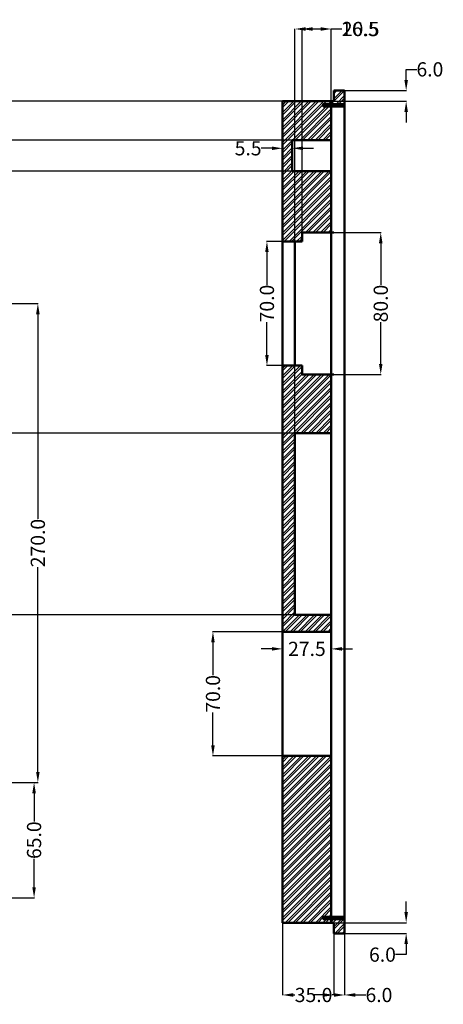
# Model space of a CAD drawing. Units: inches. Extents: x 11765 to 12471, y 10149 to 10793.
# Tile 8 of 8: x 12232 to 12471, y 10197 to 10752. Entities that reach past the tile are written whole.
import ezdxf

# ---------------------------------------------------------------- set-up
doc = ezdxf.new("R2010")
doc.units = ezdxf.units.IN
doc.header["$MEASUREMENT"] = 0
for name, color, linetype, lineweight in [('M-DIMS', 2, 'Continuous', 25), ('M-HATC', 8, 'Continuous', 18), ('M-OUTL', 7, 'Continuous', 50)]:
    doc.layers.add(name, color=color, linetype=linetype, lineweight=lineweight)
doc.styles.get("Standard").update_dxf_attribs({"font": 'arial.ttf'})
doc.dimstyles.get("Standard").update_dxf_attribs({"dimtxt": 8, "dimasz": 6, "dimexe": 0.18, "dimexo": 0.0625, "dimgap": 0.09, "dimtad": 0, "dimtoh": 1, "dimdec": 1, "dimzin": 0, "dimdsep": 46, "dimtxsty": 'Standard', "dimcen": 0.09, "dimadec": 0, "dimazin": 0, "dimtfac": 1, "dimtdec": 1, "dimtofl": 0, "dimtmove": 0, "dimatfit": 3, "dimfxl": 1, "dimtolj": 1, "dimtzin": 0, "dimarcsym": 0})

# ---------------------------------------------------------------- blocks, each defined once
blk = doc.blocks.new('*D15')
at = {"layer": 'Defpoints', "color": 0, "transparency": 16777216}
for p in [(12198.7, 10592.15), (12090.75, 10322.15), (12241.87, 10322.15)]:
    blk.add_point(p, dxfattribs=at)
at = {"layer": 'M-DIMS', "color": 0, "lineweight": -2, "transparency": 16777216}
for p, q in [((12198.76, 10592.15), (12242.05, 10592.15)), ((12241.87, 10586.15), (12241.87, 10470.79)), ((12241.87, 10328.15), (12241.87, 10443.5)), ((12090.81, 10322.15), (12242.05, 10322.15))]:
    blk.add_line(p, q, dxfattribs=at)
at = {"layer": 'M-DIMS', "color": 0, "transparency": 16777216}
for points in [[(12240.87, 10586.15), (12242.87, 10586.15), (12241.87, 10592.15)], [(12240.87, 10328.15), (12242.87, 10328.15), (12241.87, 10322.15)]]:
    blk.add_solid(points, dxfattribs=at)
at = {"layer": 'M-DIMS', "color": 0, "transparency": 16777216, "insert": (12241.87, 10457.15), "char_height": 8, "attachment_point": 5, "rotation": 90}
blk.add_mtext('\\A1;270.0', dxfattribs=at)
blk = doc.blocks.new('*D16')
at = {"layer": 'Defpoints', "color": 0, "transparency": 16777216}
for p in [(12136.92, 10322.15), (12136.92, 10257.15), (12239.74, 10257.15)]:
    blk.add_point(p, dxfattribs=at)
at = {"layer": 'M-DIMS', "color": 0, "lineweight": -2, "transparency": 16777216}
for p, q in [((12136.98, 10322.15), (12239.92, 10322.15)), ((12239.74, 10316.15), (12239.74, 10300.13)), ((12239.74, 10263.15), (12239.74, 10279.16)), ((12136.98, 10257.15), (12239.92, 10257.15))]:
    blk.add_line(p, q, dxfattribs=at)
at = {"layer": 'M-DIMS', "color": 0, "transparency": 16777216}
for points in [[(12238.74, 10316.15), (12240.74, 10316.15), (12239.74, 10322.15)], [(12238.74, 10263.15), (12240.74, 10263.15), (12239.74, 10257.15)]]:
    blk.add_solid(points, dxfattribs=at)
at = {"layer": 'M-DIMS', "color": 0, "transparency": 16777216, "insert": (12239.74, 10289.65), "char_height": 8, "attachment_point": 5, "rotation": 90}
blk.add_mtext('\\A1;65.0', dxfattribs=at)
blk = doc.blocks.new('*D53')
at = {"layer": 'Defpoints', "color": 0, "transparency": 16777216}
for p in [(12408.9, 10632.15), (12408.9, 10552.15), (12435.31, 10552.15)]:
    blk.add_point(p, dxfattribs=at)
at = {"layer": 'M-DIMS', "color": 0, "lineweight": -2, "transparency": 16777216}
for p, q in [((12408.96, 10632.15), (12435.49, 10632.15)), ((12435.31, 10626.15), (12435.31, 10602.62)), ((12435.31, 10558.15), (12435.31, 10581.67)), ((12408.96, 10552.15), (12435.49, 10552.15))]:
    blk.add_line(p, q, dxfattribs=at)
at = {"layer": 'M-DIMS', "color": 0, "transparency": 16777216}
for points in [[(12434.31, 10626.15), (12436.31, 10626.15), (12435.31, 10632.15)], [(12434.31, 10558.15), (12436.31, 10558.15), (12435.31, 10552.15)]]:
    blk.add_solid(points, dxfattribs=at)
at = {"layer": 'M-DIMS', "color": 0, "transparency": 16777216, "insert": (12435.31, 10592.15), "char_height": 8, "attachment_point": 5, "rotation": 90}
blk.add_mtext('\\A1;80.0', dxfattribs=at)
blk = doc.blocks.new('*D54')
at = {"layer": 'Defpoints', "color": 0, "transparency": 16777216}
for p in [(12379.9, 10627.15), (12371.1, 10557.15), (12379.9, 10557.15)]:
    blk.add_point(p, dxfattribs=at)
at = {"layer": 'M-DIMS', "color": 0, "lineweight": -2, "transparency": 16777216}
for p, q in [((12379.83, 10627.15), (12370.92, 10627.15)), ((12371.1, 10621.15), (12371.1, 10602.58)), ((12371.1, 10563.15), (12371.1, 10581.71)), ((12379.83, 10557.15), (12370.92, 10557.15))]:
    blk.add_line(p, q, dxfattribs=at)
at = {"layer": 'M-DIMS', "color": 0, "transparency": 16777216}
for points in [[(12370.1, 10621.15), (12372.1, 10621.15), (12371.1, 10627.15)], [(12370.1, 10563.15), (12372.1, 10563.15), (12371.1, 10557.15)]]:
    blk.add_solid(points, dxfattribs=at)
at = {"layer": 'M-DIMS', "color": 0, "transparency": 16777216, "insert": (12371.1, 10592.15), "char_height": 8, "attachment_point": 5, "rotation": 90}
blk.add_mtext('\\A1;70.0', dxfattribs=at)
blk = doc.blocks.new('*D55')
at = {"layer": 'Defpoints', "color": 0, "transparency": 16777216}
for p in [(12379.9, 10407.15), (12340.65, 10337.15), (12379.9, 10337.15)]:
    blk.add_point(p, dxfattribs=at)
at = {"layer": 'M-DIMS', "color": 0, "lineweight": -2, "transparency": 16777216}
for p, q in [((12379.83, 10407.15), (12340.47, 10407.15)), ((12340.65, 10401.15), (12340.65, 10382.58)), ((12340.65, 10343.15), (12340.65, 10361.71)), ((12379.83, 10337.15), (12340.47, 10337.15))]:
    blk.add_line(p, q, dxfattribs=at)
at = {"layer": 'M-DIMS', "color": 0, "transparency": 16777216}
for points in [[(12339.65, 10401.15), (12341.65, 10401.15), (12340.65, 10407.15)], [(12339.65, 10343.15), (12341.65, 10343.15), (12340.65, 10337.15)]]:
    blk.add_solid(points, dxfattribs=at)
at = {"layer": 'M-DIMS', "color": 0, "transparency": 16777216, "insert": (12340.65, 10372.15), "char_height": 8, "attachment_point": 5, "rotation": 90}
blk.add_mtext('\\A1;70.0', dxfattribs=at)
blk = doc.blocks.new('*D56')
at = {"layer": 'Defpoints', "color": 0, "transparency": 16777216}
for p in [(12379.9, 10679.66), (12379.9, 10678.3), (12385.4, 10678.3)]:
    blk.add_point(p, dxfattribs=at)
at = {"layer": 'M-DIMS', "color": 0, "lineweight": -2, "transparency": 16777216}
for p, q in [((12373.9, 10679.66), (12367.9, 10679.66)), ((12379.9, 10678.37), (12379.9, 10679.84)), ((12385.4, 10678.37), (12385.4, 10679.84)), ((12391.4, 10679.66), (12397.4, 10679.66))]:
    blk.add_line(p, q, dxfattribs=at)
at = {"layer": 'M-DIMS', "color": 0, "transparency": 16777216}
for points in [[(12373.9, 10680.66), (12373.9, 10678.66), (12379.9, 10679.66)], [(12391.4, 10680.66), (12391.4, 10678.66), (12385.4, 10679.66)]]:
    blk.add_solid(points, dxfattribs=at)
at = {"layer": 'M-DIMS', "color": 0, "transparency": 16777216, "insert": (12360.49, 10679.66), "char_height": 8, "attachment_point": 5}
blk.add_mtext('\\A1;5.5', dxfattribs=at)
blk = doc.blocks.new('*D57')
at = {"layer": 'Defpoints', "color": 0, "transparency": 16777216}
for p in [(12379.9, 10402.14), (12407.4, 10402.14), (12407.4, 10397.49)]:
    blk.add_point(p, dxfattribs=at)
at = {"layer": 'M-DIMS', "color": 0, "lineweight": -2, "transparency": 16777216}
for p, q in [((12379.9, 10402.07), (12379.9, 10397.31)), ((12407.4, 10402.07), (12407.4, 10397.31)), ((12373.9, 10397.49), (12367.9, 10397.49)), ((12413.4, 10397.49), (12419.4, 10397.49))]:
    blk.add_line(p, q, dxfattribs=at)
at = {"layer": 'M-DIMS', "color": 0, "transparency": 16777216}
for points in [[(12373.9, 10398.49), (12373.9, 10396.49), (12379.9, 10397.49)], [(12413.4, 10398.49), (12413.4, 10396.49), (12407.4, 10397.49)]]:
    blk.add_solid(points, dxfattribs=at)
at = {"layer": 'M-DIMS', "color": 0, "transparency": 16777216, "insert": (12393.65, 10397.49), "char_height": 8, "attachment_point": 5}
blk.add_mtext('\\A1;27.5', dxfattribs=at)
blk = doc.blocks.new('*D58')
at = {"layer": 'Defpoints', "color": 0, "transparency": 16777216}
for p in [(12379.9, 10243.15), (12414.9, 10237.15), (12414.9, 10202.4)]:
    blk.add_point(p, dxfattribs=at)
at = {"layer": 'M-DIMS', "color": 0, "lineweight": -2, "transparency": 16777216}
for p, q in [((12379.9, 10243.08), (12379.9, 10202.22)), ((12414.9, 10237.08), (12414.9, 10202.22)), ((12385.9, 10202.4), (12386.93, 10202.4)), ((12408.9, 10202.4), (12407.86, 10202.4))]:
    blk.add_line(p, q, dxfattribs=at)
at = {"layer": 'M-DIMS', "color": 0, "transparency": 16777216}
for points in [[(12385.9, 10203.4), (12385.9, 10201.4), (12379.9, 10202.4)], [(12408.9, 10203.4), (12408.9, 10201.4), (12414.9, 10202.4)]]:
    blk.add_solid(points, dxfattribs=at)
at = {"layer": 'M-DIMS', "color": 0, "transparency": 16777216, "insert": (12397.4, 10202.4), "char_height": 8, "attachment_point": 5}
blk.add_mtext('\\A1;35.0', dxfattribs=at)
blk = doc.blocks.new('*D59')
at = {"layer": 'Defpoints', "color": 0, "transparency": 16777216}
for p in [(12408.9, 10237.15), (12414.9, 10237.15), (12414.9, 10202.4)]:
    blk.add_point(p, dxfattribs=at)
at = {"layer": 'M-DIMS', "color": 0, "lineweight": -2, "transparency": 16777216}
for p, q in [((12408.9, 10237.08), (12408.9, 10202.22)), ((12414.9, 10237.08), (12414.9, 10202.22)), ((12402.9, 10202.4), (12396.9, 10202.4)), ((12420.9, 10202.4), (12426.9, 10202.4))]:
    blk.add_line(p, q, dxfattribs=at)
at = {"layer": 'M-DIMS', "color": 0, "transparency": 16777216}
for points in [[(12402.9, 10203.4), (12402.9, 10201.4), (12408.9, 10202.4)], [(12420.9, 10203.4), (12420.9, 10201.4), (12414.9, 10202.4)]]:
    blk.add_solid(points, dxfattribs=at)
at = {"layer": 'M-DIMS', "color": 0, "transparency": 16777216, "insert": (12434.28, 10202.4), "char_height": 8, "attachment_point": 5}
blk.add_mtext('\\A1;6.0', dxfattribs=at)
blk = doc.blocks.new('*D60')
at = {"layer": 'Defpoints', "color": 0, "transparency": 16777216}
for p in [(12414.9, 10712.15), (12449.65, 10712.15), (12407.4, 10706.15)]:
    blk.add_point(p, dxfattribs=at)
at = {"layer": 'M-DIMS', "color": 0, "lineweight": -2, "transparency": 16777216}
for p, q in [((12449.65, 10718.15), (12449.65, 10724.15)), ((12449.65, 10724.15), (12455.65, 10724.15)), ((12414.96, 10712.15), (12449.83, 10712.15)), ((12407.46, 10706.15), (12449.83, 10706.15)), ((12449.65, 10700.15), (12449.65, 10694.15))]:
    blk.add_line(p, q, dxfattribs=at)
at = {"layer": 'M-DIMS', "color": 0, "transparency": 16777216}
for points in [[(12448.65, 10718.15), (12450.65, 10718.15), (12449.65, 10712.15)], [(12448.65, 10700.15), (12450.65, 10700.15), (12449.65, 10706.15)]]:
    blk.add_solid(points, dxfattribs=at)
at = {"layer": 'M-DIMS', "color": 0, "transparency": 16777216, "insert": (12463.03, 10724.15), "char_height": 8, "attachment_point": 5}
blk.add_mtext('\\A1;6.0', dxfattribs=at)
blk = doc.blocks.new('*D61')
at = {"layer": 'Defpoints', "color": 0, "transparency": 16777216}
for p in [(12407.4, 10243.15), (12408.9, 10237.15), (12449.65, 10237.15)]:
    blk.add_point(p, dxfattribs=at)
at = {"layer": 'M-DIMS', "color": 0, "lineweight": -2, "transparency": 16777216}
for p, q in [((12449.65, 10249.15), (12449.65, 10255.15)), ((12407.46, 10243.15), (12449.83, 10243.15)), ((12408.96, 10237.15), (12449.83, 10237.15)), ((12449.65, 10231.15), (12449.65, 10225.15)), ((12449.65, 10225.15), (12443.65, 10225.15))]:
    blk.add_line(p, q, dxfattribs=at)
at = {"layer": 'M-DIMS', "color": 0, "transparency": 16777216}
for points in [[(12448.65, 10249.15), (12450.65, 10249.15), (12449.65, 10243.15)], [(12448.65, 10231.15), (12450.65, 10231.15), (12449.65, 10237.15)]]:
    blk.add_solid(points, dxfattribs=at)
at = {"layer": 'M-DIMS', "color": 0, "transparency": 16777216, "insert": (12436.27, 10225.15), "char_height": 8, "attachment_point": 5}
blk.add_mtext('\\A1;6.0', dxfattribs=at)
blk = doc.blocks.new('*D62')
at = {"layer": 'Defpoints', "color": 0, "transparency": 16777216}
for p in [(12379.9, 10706.15), (11848.16, 10684.29), (12385.4, 10684.29)]:
    blk.add_point(p, dxfattribs=at)
at = {"layer": 'M-DIMS', "color": 0, "lineweight": -2, "transparency": 16777216}
for p, q in [((12379.83, 10706.15), (11847.98, 10706.15)), ((11848.16, 10700.15), (11848.16, 10690.29)), ((12385.33, 10684.29), (11847.98, 10684.29)), ((11848.16, 10684.29), (11848.16, 10678.29)), ((11848.16, 10678.29), (11842.16, 10678.29))]:
    blk.add_line(p, q, dxfattribs=at)
at = {"layer": 'M-DIMS', "color": 0, "transparency": 16777216}
for points in [[(11847.16, 10700.15), (11849.16, 10700.15), (11848.16, 10706.15)], [(11847.16, 10690.29), (11849.16, 10690.29), (11848.16, 10684.29)]]:
    blk.add_solid(points, dxfattribs=at)
at = {"layer": 'M-DIMS', "color": 0, "transparency": 16777216, "insert": (11828.51, 10678.29), "char_height": 8, "attachment_point": 5}
blk.add_mtext('\\A1;21.86', dxfattribs=at)
blk = doc.blocks.new('*D63')
at = {"layer": 'Defpoints', "color": 0, "transparency": 16777216}
for p in [(12385.4, 10684.29), (11848.16, 10666.79), (12385.4, 10666.79)]:
    blk.add_point(p, dxfattribs=at)
at = {"layer": 'M-DIMS', "color": 0, "lineweight": -2, "transparency": 16777216}
for p, q in [((12385.33, 10684.29), (11847.98, 10684.29)), ((11848.16, 10678.29), (11848.16, 10672.79)), ((12385.33, 10666.79), (11847.98, 10666.79)), ((11848.16, 10666.79), (11848.16, 10660.79)), ((11848.16, 10660.79), (11842.16, 10660.79))]:
    blk.add_line(p, q, dxfattribs=at)
at = {"layer": 'M-DIMS', "color": 0, "transparency": 16777216}
for points in [[(11847.16, 10678.29), (11849.16, 10678.29), (11848.16, 10684.29)], [(11847.16, 10672.79), (11849.16, 10672.79), (11848.16, 10666.79)]]:
    blk.add_solid(points, dxfattribs=at)
at = {"layer": 'M-DIMS', "color": 0, "transparency": 16777216, "insert": (11832.03, 10660.79), "char_height": 8, "attachment_point": 5}
blk.add_mtext('\\A1;17.5', dxfattribs=at)
blk = doc.blocks.new('*D64')
at = {"layer": 'Defpoints', "color": 0, "transparency": 16777216}
for p in [(12407.4, 10746.9), (12390.9, 10632.15), (12407.4, 10519.15)]:
    blk.add_point(p, dxfattribs=at)
at = {"layer": 'M-DIMS', "color": 0, "lineweight": -2, "transparency": 16777216}
for p, q in [((12390.9, 10632.21), (12390.9, 10747.08)), ((12396.9, 10746.9), (12401.4, 10746.9)), ((12407.4, 10519.21), (12407.4, 10747.08)), ((12407.4, 10746.9), (12413.4, 10746.9))]:
    blk.add_line(p, q, dxfattribs=at)
at = {"layer": 'M-DIMS', "color": 0, "transparency": 16777216}
for points in [[(12396.9, 10747.9), (12396.9, 10745.9), (12390.9, 10746.9)], [(12401.4, 10747.9), (12401.4, 10745.9), (12407.4, 10746.9)]]:
    blk.add_solid(points, dxfattribs=at)
at = {"layer": 'M-DIMS', "color": 0, "transparency": 16777216, "insert": (12423.53, 10746.9), "char_height": 8, "attachment_point": 5}
blk.add_mtext('\\A1;16.5', dxfattribs=at)
blk = doc.blocks.new('*D65')
at = {"layer": 'Defpoints', "color": 0, "transparency": 16777216}
for p in [(12407.4, 10746.9), (12386.9, 10519.15), (12407.4, 10519.15)]:
    blk.add_point(p, dxfattribs=at)
at = {"layer": 'M-DIMS', "color": 0, "lineweight": -2, "transparency": 16777216}
for p, q in [((12386.9, 10519.21), (12386.9, 10747.08)), ((12392.9, 10746.9), (12401.4, 10746.9)), ((12407.4, 10519.21), (12407.4, 10747.08)), ((12407.4, 10746.9), (12413.4, 10746.9))]:
    blk.add_line(p, q, dxfattribs=at)
at = {"layer": 'M-DIMS', "color": 0, "transparency": 16777216}
for points in [[(12392.9, 10747.9), (12392.9, 10745.9), (12386.9, 10746.9)], [(12401.4, 10747.9), (12401.4, 10745.9), (12407.4, 10746.9)]]:
    blk.add_solid(points, dxfattribs=at)
at = {"layer": 'M-DIMS', "color": 0, "transparency": 16777216, "insert": (12423.97, 10746.9), "char_height": 8, "attachment_point": 5}
blk.add_mtext('\\A1;20.5', dxfattribs=at)
blk = doc.blocks.new('*D66')
at = {"layer": 'Defpoints', "color": 0, "transparency": 16777216}
for p in [(12386.9, 10519.15), (11848.16, 10416.65), (12386.9, 10416.65)]:
    blk.add_point(p, dxfattribs=at)
at = {"layer": 'M-DIMS', "color": 0, "lineweight": -2, "transparency": 16777216}
for p, q in [((12386.83, 10519.15), (11847.98, 10519.15)), ((11848.16, 10513.15), (11848.16, 10481.14)), ((11848.16, 10422.65), (11848.16, 10454.65)), ((12386.83, 10416.65), (11847.98, 10416.65))]:
    blk.add_line(p, q, dxfattribs=at)
at = {"layer": 'M-DIMS', "color": 0, "transparency": 16777216}
for points in [[(11847.16, 10513.15), (11849.16, 10513.15), (11848.16, 10519.15)], [(11847.16, 10422.65), (11849.16, 10422.65), (11848.16, 10416.65)]]:
    blk.add_solid(points, dxfattribs=at)
at = {"layer": 'M-DIMS', "color": 0, "transparency": 16777216, "insert": (11848.16, 10467.9), "char_height": 8, "attachment_point": 5, "rotation": 90}
blk.add_mtext('\\A1;102.5', dxfattribs=at)

msp = doc.modelspace()

# ---------------------------------------------------------------- hatches: boundary and pattern name
at = {"layer": 'M-HATC'}
h = msp.add_hatch(dxfattribs=at)
h.set_pattern_fill('ANSI32', color=256, scale=8, style=0)
h.paths.add_polyline_path([(12407.396, 10632.146), (12407.396, 10666.786), (12385.396, 10666.786), (12385.396, 10684.286), (12407.396, 10684.286), (12407.396, 10703.271), (12402.896, 10703.271), (12402.896, 10704.559), (12414.896, 10704.559), (12414.896, 10712.146), (12408.896, 10712.146), (12408.896, 10706.146), (12379.896, 10706.146), (12379.896, 10627.146), (12390.896, 10627.146), (12390.896, 10632.146)])
h.paths.add_polyline_path([(12407.396, 10246.441), (12407.396, 10337.146), (12379.896, 10337.146), (12379.896, 10243.146), (12408.896, 10243.146), (12408.896, 10237.146), (12414.896, 10237.146), (12414.896, 10245.153), (12402.896, 10245.153), (12402.896, 10246.441)])
h.paths.add_polyline_path([(12407.396, 10519.146), (12407.396, 10552.146), (12390.896, 10552.146), (12390.896, 10557.146), (12379.896, 10557.146), (12379.896, 10407.146), (12407.396, 10407.146), (12407.396, 10416.646), (12386.896, 10416.646), (12386.896, 10519.146)])

# ---------------------------------------------------------------- linework, layer by layer
at = {"layer": 'M-OUTL'}
for p, q in [((12408.896, 10712.146), (12414.896, 10712.146)), ((12408.896, 10712.146), (12408.896, 10706.146)), ((12408.896, 10712.146), (12408.896, 10706.146)), ((12414.896, 10712.146), (12414.896, 10237.146)), ((12379.896, 10706.146), (12379.896, 10243.146)), ((12379.896, 10706.146), (12408.896, 10706.146)), ((12407.396, 10706.146), (12407.396, 10243.146)), ((12402.896, 10704.559), (12402.896, 10703.271)), ((12385.396, 10684.286), (12407.396, 10684.286)), ((12385.396, 10684.286), (12385.396, 10666.786)), ((12385.396, 10684.286), (12385.396, 10666.786)), ((12385.396, 10666.786), (12407.396, 10666.786)), ((12390.896, 10632.146), (12408.896, 10632.146)), ((12390.896, 10632.146), (12390.896, 10627.146)), ((12379.896, 10627.146), (12390.896, 10627.146)), ((12386.896, 10627.146), (12386.896, 10557.146)), ((12379.896, 10557.146), (12390.896, 10557.146)), ((12390.896, 10557.146), (12390.896, 10552.146)), ((12390.896, 10552.146), (12408.896, 10552.146)), ((12386.896, 10519.146), (12407.396, 10519.146)), ((12386.896, 10519.146), (12386.896, 10416.646)), ((12386.896, 10416.646), (12407.396, 10416.646)), ((12379.896, 10407.146), (12407.396, 10407.146)), ((12379.896, 10337.146), (12407.396, 10337.146)), ((12402.896, 10246.441), (12402.896, 10245.153)), ((12379.896, 10243.146), (12408.896, 10243.146)), ((12408.896, 10243.146), (12408.896, 10237.146)), ((12408.896, 10237.146), (12414.896, 10237.146))]:
    msp.add_line(p, q, dxfattribs=at)
for points in [[(12414.896, 10704.559), (12402.896, 10704.559), (12402.896, 10703.271), (12414.896, 10703.271)], [(12414.896, 10246.441), (12402.896, 10246.441), (12402.896, 10245.153), (12414.896, 10245.153)]]:
    msp.add_lwpolyline(points, dxfattribs=at)

# ---------------------------------------------------------------- dimensions: what is measured, and where the dimension line sits
at = {"layer": 'M-DIMS'}
for base, p1, p2, override, picture, middle in [((12407.396, 10746.896), (12386.896, 10519.146), (12407.396, 10519.146), {"dimdec": 1, "dimlfac": 1, "dimrnd": 0, "dimzin": 0, "dimdsep": 46, "dimlunit": 2}, '*D65', (12423.975, 10746.896)), ((12407.396, 10746.896), (12390.896, 10632.146), (12407.396, 10519.146), {"dimdec": 1, "dimlfac": 1, "dimrnd": 0, "dimzin": 0, "dimdsep": 46, "dimlunit": 2}, '*D64', (12423.53, 10746.896)), ((12379.896, 10679.662), (12385.396, 10678.303), (12379.896, 10678.303), {"dimclrd": 0, "dimclre": 0, "dimclrt": 0}, '*D56', (12360.494, 10679.662)), ((12407.396, 10397.487), (12379.896, 10402.137), (12407.396, 10402.137), {"dimclrd": 0, "dimclre": 0, "dimclrt": 0}, '*D57', (12393.646, 10397.487)), ((12414.896, 10202.396), (12379.896, 10243.146), (12414.896, 10237.146), {"dimdec": 1, "dimlfac": 1, "dimrnd": 0, "dimzin": 0, "dimdsep": 46, "dimlunit": 2}, '*D58', (12397.396, 10202.396)), ((12414.896, 10202.396), (12408.896, 10237.146), (12414.896, 10237.146), {"dimdec": 1, "dimlfac": 1, "dimrnd": 0, "dimzin": 0, "dimdsep": 46, "dimlunit": 2}, '*D59', (12434.277, 10202.396))]:
    dim = msp.add_linear_dim(base=base, p1=p1, p2=p2, dimstyle='Standard', override=override, dxfattribs=at)
    dim.commit()
    dim.dimension.update_dxf_attribs({"geometry": picture, "text_midpoint": middle})
for base, p1, p2, override, picture, middle in [((12449.646, 10712.146), (12407.396, 10706.146), (12414.896, 10712.146), {"dimdec": 1, "dimlfac": 1, "dimrnd": 0, "dimzin": 0, "dimdsep": 46, "dimlunit": 2}, '*D60', (12463.027, 10724.146)), ((11848.162, 10684.286), (12379.896, 10706.146), (12385.396, 10684.286), {"dimdec": 2, "dimlfac": 1, "dimrnd": 0, "dimzin": 0, "dimdsep": 46, "dimlunit": 2}, '*D62', (11828.509, 10678.286)), ((11848.162, 10666.786), (12385.396, 10684.286), (12385.396, 10666.786), {"dimdec": 1, "dimlfac": 1, "dimrnd": 0, "dimzin": 0, "dimdsep": 46, "dimlunit": 2}, '*D63', (11832.028, 10660.786)), ((12435.305, 10552.146), (12408.896, 10632.146), (12408.896, 10552.146), {"dimclrd": 0, "dimclre": 0, "dimclrt": 0}, '*D53', (12435.305, 10592.146)), ((12371.101, 10557.146), (12379.896, 10627.146), (12379.896, 10557.146), {"dimclrd": 0, "dimclre": 0, "dimclrt": 0}, '*D54', (12371.101, 10592.146)), ((12241.874, 10322.146), (12198.696, 10592.146), (12090.748, 10322.146), {"dimclrd": 0, "dimclre": 0, "dimclrt": 0}, '*D15', (12241.874, 10457.146)), ((11848.162, 10416.646), (12386.896, 10519.146), (12386.896, 10416.646), {"dimdec": 1, "dimlfac": 1, "dimrnd": 0, "dimzin": 0, "dimdsep": 46, "dimlunit": 2}, '*D66', (11848.162, 10467.896)), ((12340.652, 10337.146), (12379.896, 10407.146), (12379.896, 10337.146), {"dimclrd": 0, "dimclre": 0, "dimclrt": 0}, '*D55', (12340.652, 10372.146)), ((12239.736, 10257.146), (12136.919, 10322.146), (12136.919, 10257.146), {"dimclrd": 0, "dimclre": 0, "dimclrt": 0}, '*D16', (12239.736, 10289.646)), ((12449.646, 10237.146), (12407.396, 10243.146), (12408.896, 10237.146), {"dimdec": 1, "dimlfac": 1, "dimrnd": 0, "dimzin": 0, "dimdsep": 46, "dimlunit": 2}, '*D61', (12436.266, 10225.146))]:
    dim = msp.add_linear_dim(base=base, p1=p1, p2=p2, angle=90, dimstyle='Standard', override=override, dxfattribs=at)
    dim.commit()
    dim.dimension.update_dxf_attribs({"geometry": picture, "text_midpoint": middle})

doc.saveas('drawing.dxf')
